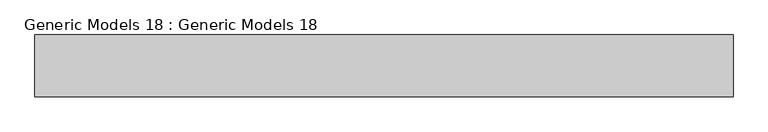
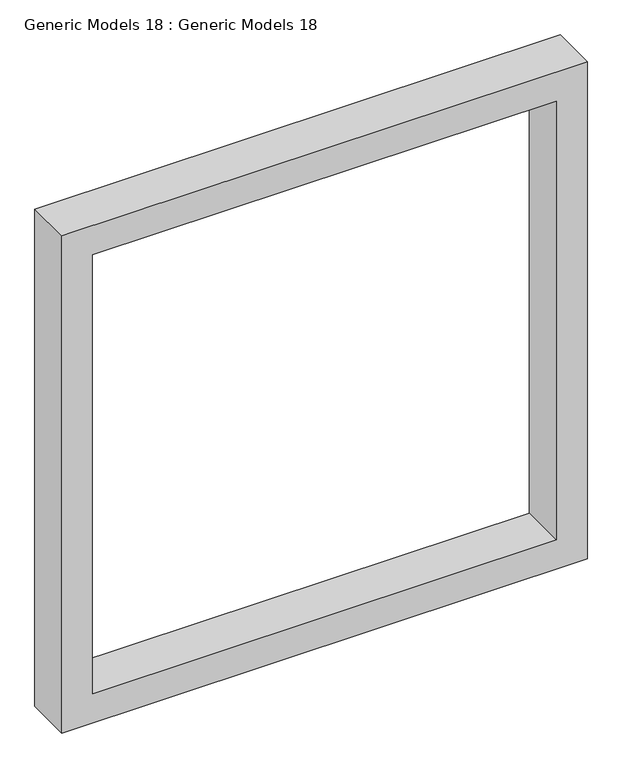
"""IFC4 building model written with IfcOpenShell, lengths in millimetres: proxy geometry, Generic Models 18 : Generic Models 18."""

from ifc_helpers import new_model, si_unit, frame, origin, place, context, project, spatial, polyline, outline, extrude, source, transform, mapped, element, save


def generic_models_18_generic_models_18_bc45088a(model_context):
    return source(origin(), model_context, "Body", "SweptSolid", [
        extrude(outline(polyline([(8940.8, -903.1280307), (7213.6, -903.1280307), (7213.6, 824.0719693), (8940.8, 824.0719693), (8940.8, -903.1280307)]), holes=[polyline([(8839.2, -801.5280307), (8839.2, 722.4719693), (7315.2, 722.4719693), (7315.2, -801.5280307), (8839.2, -801.5280307)])]), frame((0.0, 12268.2641252, 0.0), z_axis=(0.0, 1.0, 0.0), x_axis=(0.0, 0.0, 1.0)), (0.0, 0.0, 1.0), 152.4),
    ])


if __name__ == "__main__":
    model = new_model("IFC4")
    model_context = context("Model", 3, world=origin())
    ifc_project = project(units=[si_unit("LENGTHUNIT", "METRE", prefix="MILLI")], contexts=[model_context])
    site = spatial("IfcSite", under=ifc_project)
    building = spatial("IfcBuilding", under=site)
    placement = place(None, origin())
    generic_models_18_generic_models_18_shape = generic_models_18_generic_models_18_bc45088a(model_context)
    element("IfcBuildingElementProxy", 1, Name="Generic Models 18 : Generic Models 18", ObjectType="Generic Models 18 : Generic Models 18", at=placement, inside=building, context=model_context, shape_type="MappedRepresentation", body=[
        mapped(generic_models_18_generic_models_18_shape, transform((0.0, 0.0, 0.0), x_axis=(1.0, 0.0, 0.0), y_axis=(0.0, 1.0, 0.0), z_axis=(0.0, 0.0, 1.0))),
    ])
    save(model, "model.ifc")

# Revit data of these elements
# Element 1 (IfcBuildingElementProxy, "Generic Models 18 : Generic Models 18")
#   Materials on its faces: "chocolate brown"
# Materials
#   "chocolate brown": class "Generic", colour RGB 120 120 120, transparency 0, Cost = 0
